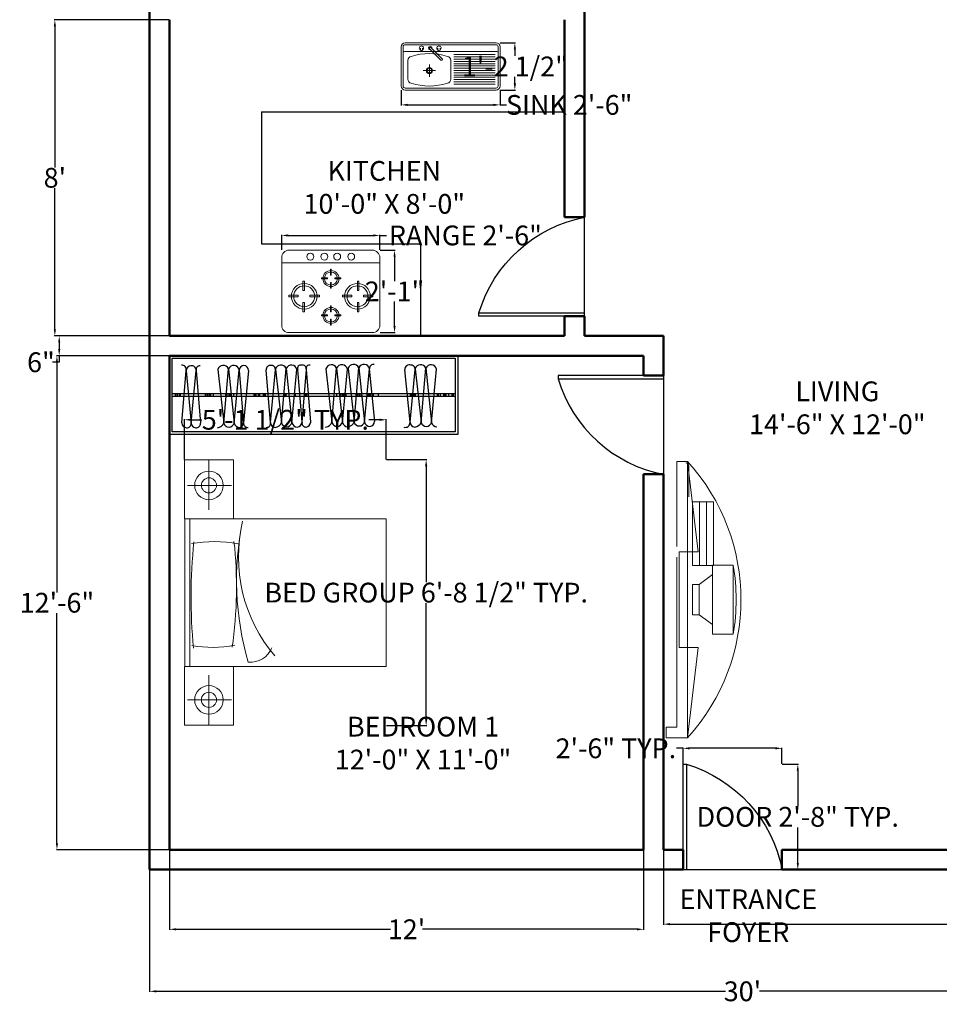
# Model space of a CAD drawing. Units: inches. Extents: x 20 to 32681, y 45 to 3082.
# Tile 1 of 5: x 21 to 301, y 45 to 344. Entities that reach past the tile are written whole.
import ezdxf

# ---------------------------------------------------------------- set-up
doc = ezdxf.new("R2010")
doc.units = ezdxf.units.IN
doc.header["$MEASUREMENT"] = 0
for name, color, linetype, lineweight in [('A-ANNO-DIMS', 2, 'Continuous', 18), ('A-AREA-IDEN', 7, 'Continuous', 25), ('A-DOOR', 4, 'Continuous', 25), ('A-EQPM', 9, 'Continuous', 18), ('A-FLOR-CASE', 32, 'Continuous', 25), ('A-FLOR-FIXT', 8, 'Continuous', 18), ('A-FURN', 8, 'Continuous', 18), ('A-WALL', 7, 'Continuous', 50)]:
    doc.layers.add(name, color=color, linetype=linetype, lineweight=lineweight)
doc.styles.get("Standard").update_dxf_attribs({"font": 'arial.ttf'})
doc.dimstyles.get("Standard").update_dxf_attribs({"dimtxt": 6, "dimasz": 2, "dimexe": 0.18, "dimexo": 0.0625, "dimgap": 0.09, "dimtad": 0, "dimtih": 1, "dimtoh": 1, "dimdec": 0, "dimzin": 0, "dimdsep": 46, "dimlunit": 4, "dimtxsty": 'Standard', "dimcen": 0.09, "dimadec": 0, "dimazin": 0, "dimtfac": 1, "dimtdec": 0, "dimtofl": 0, "dimtmove": 0, "dimatfit": 3, "dimfxl": 1, "dimtolj": 1, "dimtzin": 0, "dimarcsym": 0})

# ---------------------------------------------------------------- blocks, each defined once
blk = doc.blocks.new('DOOR')
for p, q in [((234.79, 441.58), (233.79, 441.58)), ((233.79, 441.58), (233.79, 409.58)), ((234.79, 409.58), (234.79, 441.58)), ((234.79, 409.58), (204.79, 409.58))]:
    blk.add_line(p, q)
blk.add_arc((245.82, 401.53), 41.82, 106.7253, 168.9058)
blk = doc.blocks.new('CVBN')
for p, q in [((70.94, 1179.16), (70.94, 1191.01)), ((89.36, 1192.66), (89.36, 1168.36)), ((89.36, 1081.69), (89.36, 1192.39)), ((89.36, 1192.39), (89.36, 1168.09)), ((170.36, 1192.39), (89.36, 1192.39)), ((170.36, 1192.66), (170.36, 1168.36)), ((170.36, 1081.69), (170.36, 1192.39)), ((170.36, 1192.39), (170.36, 1168.09)), ((170.36, 1192.39), (170.36, 1168.09)), ((188.79, 1179.16), (188.79, 1191.01)), ((170.36, 1189.69), (89.36, 1189.69)), ((70.94, 1179.16), (56.8, 1179.16)), ((70.94, 1179.16), (84.43, 1179.16)), ((70.94, 1179.16), (70.94, 1166.85)), ((188.79, 1179.16), (175.29, 1179.16)), ((188.79, 1179.16), (202.93, 1179.16)), ((188.79, 1179.16), (188.79, 1166.85)), ((170.36, 1081.69), (89.36, 1081.69))]:
    blk.add_line(p, q)
for points in [[(56.96, 1192.66), (56.96, 1165.66), (89.36, 1165.66), (89.36, 1192.66)], [(202.76, 1192.66), (202.76, 1165.66), (170.36, 1165.66), (170.36, 1192.66)]]:
    blk.add_lwpolyline(points, close=True)
for centre, radius in [((70.94, 1179.16), 7.85), ((188.79, 1179.16), 7.85), ((70.94, 1179.16), 4.15), ((188.79, 1179.16), 4.15)]:
    blk.add_circle(centre, radius)
for centre, radius, start, end in [((127.34, 900.05), 288.94, 83.953, 95.5626), ((165.23, 1177.16), 65.44, 169.9145, 190.6851), ((88.06, 1176.29), 69.84, 349.1761, 10.2706), ((136.55, 1004.48), 159.53, 78.2462, 106.3473), ((132.8, 1394.24), 230.23, 261.7649, 276.2896), ((149.51, 1078.87), 84.09, 76.5636, 130.3236), ((104.49, 1156.51), 12.88, 175.3269, 247.5588)]:
    blk.add_arc(centre, radius, start, end)
blk = doc.blocks.new('A$C025C2FF6')
for p, q in [((45, 500), (550, 500)), ((0, 45), (0, 455)), ((295.2, 454.2), (300.9, 454.2)), ((295.2, 418.5), (295.2, 454.2)), ((300.9, 418.5), (295.2, 418.5)), ((300.9, 454.2), (300.9, 418.5)), ((595, 455), (595, 45)), ((128.2, 316.3), (128.2, 373.4)), ((128.2, 373.4), (137.4, 373.4)), ((137.4, 373.4), (137.4, 316.3)), ((241.9, 397.2), (241.9, 391.5)), ((277.6, 397.2), (241.9, 397.2)), ((241.9, 391.5), (277.6, 391.5)), ((277.6, 391.5), (277.6, 397.2)), ((295.2, 374), (295.2, 338.4)), ((300.9, 374), (295.2, 374)), ((300.9, 338.4), (300.9, 374)), ((322.1, 397.2), (357.7, 397.2)), ((322.1, 391.5), (322.1, 397.2)), ((357.7, 391.5), (322.1, 391.5)), ((357.7, 397.2), (357.7, 391.5)), ((467.8, 373.4), (458.7, 373.4)), ((458.7, 373.4), (458.7, 316.3)), ((467.8, 316.3), (467.8, 373.4)), ((137.4, 316.3), (128.2, 316.3)), ((295.2, 338.4), (300.9, 338.4)), ((458.7, 316.3), (467.8, 316.3)), ((100.1, 282.2), (43, 282.2)), ((43, 282.2), (43, 273.1)), ((43, 273.1), (100.1, 273.1)), ((100.1, 273.1), (100.1, 282.2)), ((128.2, 245.2), (128.2, 188.1)), ((137.4, 245.2), (128.2, 245.2)), ((137.4, 188.1), (137.4, 245.2)), ((171.3, 282.2), (228.3, 282.2)), ((171.3, 273.1), (171.3, 282.2)), ((228.3, 273.1), (171.3, 273.1)), ((228.3, 282.2), (228.3, 273.1)), ((367.8, 282.2), (367.8, 273.1)), ((424.8, 282.2), (367.8, 282.2)), ((367.8, 273.1), (424.8, 273.1)), ((424.8, 273.1), (424.8, 282.2)), ((458.7, 188.1), (458.7, 245.2)), ((458.7, 245.2), (467.8, 245.2)), ((467.8, 245.2), (467.8, 188.1)), ((496, 273.1), (496, 282.2)), ((496, 282.2), (553, 282.2)), ((553, 273.1), (496, 273.1)), ((553, 282.2), (553, 273.1)), ((128.2, 188.1), (137.4, 188.1)), ((295.2, 195.2), (295.2, 230.9)), ((295.2, 230.9), (300.9, 230.9)), ((300.9, 195.2), (295.2, 195.2)), ((300.9, 230.9), (300.9, 195.2)), ((467.8, 188.1), (458.7, 188.1)), ((277.6, 173.9), (241.9, 173.9)), ((241.9, 173.9), (241.9, 168.2)), ((241.9, 168.2), (277.6, 168.2)), ((277.6, 168.2), (277.6, 173.9)), ((300.9, 150.7), (295.2, 150.7)), ((295.2, 150.7), (295.2, 115.1)), ((300.9, 115.1), (300.9, 150.7)), ((322.1, 168.2), (322.1, 173.9)), ((322.1, 173.9), (357.7, 173.9)), ((357.7, 168.2), (322.1, 168.2)), ((357.7, 173.9), (357.7, 168.2)), ((1.2, 76.7), (594.9, 76.7)), ((295.2, 115.1), (300.9, 115.1)), ((550, 0), (45, 0))]:
    blk.add_line(p, q)
at = {"extrusion": (1e-16, 1e-16, -1)}
for centre, start_param, end_param in [((45, 455), 3.926991, 5.497787), ((550, 45), 0.785398, 2.356194)]:
    blk.add_ellipse(centre, major_axis=(31.8, 31.8), ratio=1, start_param=start_param, end_param=end_param, dxfattribs=at)
at = {"extrusion": (0, 0, -1)}
for centre, start_param, end_param in [((550, 455), 0.785398, 2.356194), ((45, 45), 3.926991, 5.497787)]:
    blk.add_ellipse(centre, major_axis=(-31.8, 31.8), ratio=1, start_param=start_param, end_param=end_param, dxfattribs=at)
at = {"extrusion": (1e-16, 3e-16, -1)}
for centre in [(298.7, 395.6), (298.7, 172.3)]:
    blk.add_ellipse(centre, major_axis=(-34.4, 34.4), ratio=1, start_param=5.497787, end_param=11.780972, dxfattribs=at)
at = {"extrusion": (1e-16, 2e-16, -1)}
for centre in [(298.7, 395.6), (298.7, 172.3)]:
    blk.add_ellipse(centre, major_axis=(-28.1, 28.1), ratio=1, start_param=5.497787, end_param=11.780972, dxfattribs=at)
at = {"extrusion": (-1e-16, -1e-16, -1)}
blk.add_ellipse((136.5, 279.7), major_axis=(-55.1, 55.1), ratio=1, start_param=5.497787, end_param=11.780972, dxfattribs=at)
at = {"extrusion": (0, -4e-16, -1)}
blk.add_ellipse((136.5, 279.7), major_axis=(-44.9, 44.9), ratio=1, start_param=5.497787, end_param=11.780972, dxfattribs=at)
for centre, major_axis, start_param, end_param in [((459.5, 279.7), (55.1, 55.1), 5.497787, 11.780972), ((459.5, 279.7), (44.9, 44.9), 5.497787, 11.780972), ((336.3, 39), (-14.8, 14.8), 3.926991, 10.210176), ((421.3, 39), (-14.8, 14.8), 3.926991, 10.210176)]:
    blk.add_ellipse(centre, major_axis=major_axis, ratio=1, start_param=start_param, end_param=end_param)
at = {"extrusion": (2e-16, -1e-16, -1)}
for centre in [(173.7, 39), (258.7, 39)]:
    blk.add_ellipse(centre, major_axis=(14.8, 14.8), ratio=1, start_param=3.926991, end_param=10.210176, dxfattribs=at)
blk = doc.blocks.new('A$C24281843')
for p, q in [((0, 0.742), (0, 0.067)), ((1.626, 0.81), (0.067, 0.81)), ((0.067, 0.776), (1.626, 0.776)), ((0.328, 0.681), (0.328, 0.718)), ((0.366, 0.681), (0.366, 0.718)), ((0.487, 0.708), (0.681, 0.514)), ((0.701, 0.534), (0.507, 0.728)), ((0.628, 0.681), (0.628, 0.718)), ((0.666, 0.681), (0.666, 0.718)), ((1.693, 0.067), (1.693, 0.742)), ((1.637, 0.66), (0.056, 0.66)), ((0.134, 0.66), (0.056, 0.66)), ((0.115, 0.508), (0.115, 0.186)), ((0.85, 0.186), (0.85, 0.508)), ((0.902, 0.607), (1.607, 0.607)), ((0.902, 0.568), (1.607, 0.568)), ((0.902, 0.529), (1.607, 0.529)), ((0.482, 0.439), (0.482, 0.224)), ((0.902, 0.49), (1.607, 0.49)), ((0.902, 0.451), (1.607, 0.451)), ((0.902, 0.412), (1.607, 0.412)), ((0.902, 0.373), (1.607, 0.373)), ((0.375, 0.332), (0.59, 0.332)), ((0.902, 0.334), (1.607, 0.334)), ((0.902, 0.296), (1.607, 0.296)), ((0.902, 0.257), (1.607, 0.257)), ((0.902, 0.218), (1.607, 0.218)), ((0.902, 0.179), (1.607, 0.179)), ((0.067, 0.034), (1.626, 0.034)), ((0.902, 0.14), (1.607, 0.14)), ((0.902, 0.101), (1.607, 0.101)), ((1.626, 0), (0.067, 0))]:
    blk.add_line(p, q)
for points in [[(0.034, 0.742), (0.034, 0.067)], [(1.66, 0.067), (1.66, 0.742)]]:
    blk.add_lwpolyline(points)
for points in [[(0.172, 0.576, -0.154641), (0.792, 0.576)], [(0.172, 0.117, 0.154641), (0.792, 0.117, -0.022148)]]:
    blk.add_lwpolyline(points, format="xyb")
for radius in [0.0538, 0.0403]:
    blk.add_circle((0.482, 0.332), radius)
for centre, radius, start, end in [((0.067, 0.742), 0.0675, 90, 180), ((0.067, 0.742), 0.0338, 90, 180), ((0.347, 0.718), 0.0375, 300, 240), ((0.347, 0.706), 0.0318, 233.9153, 306.0847), ((0.497, 0.718), 0.0281, 345, 285), ((0.497, 0.718), 0.0141, 45, 225), ((0.647, 0.718), 0.0375, 300, 240), ((0.647, 0.706), 0.0318, 233.9153, 306.0847), ((1.626, 0.742), 0.0675, 0, 90), ((1.626, 0.742), 0.0338, 0, 90), ((0.056, 0.637), 0.0225, 90, 180), ((0.184, 0.508), 0.07, 100.6708, 179.5694), ((0.691, 0.524), 0.0141, 225, 45), ((0.78, 0.508), 0.07, 0.4306, 79.3292), ((1.637, 0.637), 0.0225, 0, 90), ((0.184, 0.186), 0.07, 180.4306, 259.3292), ((0.78, 0.186), 0.07, 280.6708, 359.5694), ((0.067, 0.067), 0.0675, 180, 270), ((0.067, 0.067), 0.0338, 180, 270), ((1.626, 0.067), 0.0675, 270, 0), ((1.626, 0.067), 0.0338, 270, 0)]:
    blk.add_arc(centre, radius, start, end)
blk = doc.blocks.new('A$C1DC223CE')
for p, q in [((0, 600, -1028.6), (2200, 600, -1028.6)), ((0, 0, -1028.6), (0, 600, -1028.6)), ((20, 580, -1028.6), (2180, 580, -1028.6)), ((20, 20, -1028.6), (20, 580, -1028.6)), ((2180, 580, -1028.6), (2180, 20, -1028.6)), ((2200, 600, -1028.6), (2200, 0, -1028.6)), ((94.7, 87.9, -1028.6), (127.5, 487.8, -1028.6)), ((127.7, 485.6, -1028.6), (166.3, 85.2, -1028.6)), ((165.4, 87.9, -1028.6), (203.9, 488.4, -1028.6)), ((203.9, 488.4, -1028.6), (236.8, 85.2, -1028.6)), ((369, 495.3, -1028.6), (414.4, 87.9, -1028.6)), ((414.4, 85.2, -1028.6), (450.2, 500.8, -1028.6)), ((450.2, 499.4, -1028.6), (494.2, 86.5, -1028.6)), ((494.2, 85.2, -1028.6), (532.8, 491.1, -1028.6)), ((532.8, 488.4, -1028.6), (565.6, 84.9, -1028.6)), ((604.3, 488.4, -1028.6), (565.8, 87.9, -1028.6)), ((770.7, 91.2, -1028.6), (737.6, 491.1, -1028.6)), ((770.7, 90.7, -1028.6), (809.2, 491.1, -1028.6)), ((809.2, 498, -1028.6), (854.6, 90.7, -1028.6)), ((854.6, 87.9, -1028.6), (890.4, 503.5, -1028.6)), ((890.4, 502.1, -1028.6), (934.4, 89.3, -1028.6)), ((934.4, 87.9, -1028.6), (973, 493.9, -1028.6)), ((1011.5, 93.4, -1028.6), (978.9, 493.9, -1028.6)), ((1011.5, 93.2, -1028.6), (1044.5, 493.9, -1028.6)), ((1077.5, 93.4, -1028.6), (1044.9, 493.9, -1028.6)), ((1193.8, 500.5, -1028.6), (1239.2, 93.1, -1028.6)), ((1239.2, 90.4, -1028.6), (1275, 506, -1028.6)), ((1275, 504.6, -1028.6), (1319, 91.8, -1028.6)), ((1319, 90.4, -1028.6), (1357.6, 496.4, -1028.6)), ((1363.1, 503.2, -1028.6), (1408.5, 95.9, -1028.6)), ((1408.5, 93.1, -1028.6), (1444.3, 508.7, -1028.6)), ((1444.3, 507.4, -1028.6), (1488.3, 94.5, -1028.6)), ((1488.3, 93.1, -1028.6), (1526.8, 499.1, -1028.6)), ((1565.4, 98.6, -1028.6), (1526.8, 499.1, -1028.6)), ((1835.1, 92.3, -1028.6), (1794.6, 493.3, -1028.6)), ((1835.1, 93.1, -1028.6), (1873.6, 493.6, -1028.6)), ((1873.6, 500.5, -1028.6), (1919, 93.1, -1028.6)), ((1919, 90.4, -1028.6), (1954.8, 506, -1028.6)), ((1954.8, 504.6, -1028.6), (1998.8, 91.8, -1028.6)), ((1998.8, 90.4, -1028.6), (2037.4, 496.4, -1028.6)), ((2180, 309.1, -1028.6), (20, 309.1, -1028.6)), ((44.6, 309.1, -1028.6), (44.6, 288.1, -1028.6)), ((50, 309.1, -1028.6), (50, 288.1, -1028.6)), ((62.8, 309.1, -1028.6), (62.8, 288.1, -1028.6)), ((77.5, 309.1, -1028.6), (77.5, 288.1, -1028.6)), ((82.9, 309.1, -1028.6), (82.9, 288.1, -1028.6)), ((272.7, 309.1, -1028.6), (272.7, 288.1, -1028.6)), ((278.2, 309.1, -1028.6), (278.2, 288.1, -1028.6)), ((291, 309.1, -1028.6), (291, 288.1, -1028.6)), ((303.7, 309.1, -1028.6), (303.7, 288.1, -1028.6)), ((312.9, 309.1, -1028.6), (312.9, 288.1, -1028.6)), ((333, 309.1, -1028.6), (333, 288.1, -1028.6)), ((427.5, 309.1, -1028.6), (427.5, 288.1, -1028.6)), ((433, 309.1, -1028.6), (433, 288.1, -1028.6)), ((445.8, 309.1, -1028.6), (445.8, 288.1, -1028.6)), ((458.6, 309.1, -1028.6), (458.6, 288.1, -1028.6)), ((467.7, 309.1, -1028.6), (467.7, 288.1, -1028.6)), ((487.8, 309.1, -1028.6), (487.8, 288.1, -1028.6)), ((644.9, 309.1, -1028.6), (644.9, 288.1, -1028.6)), ((650.4, 309.1, -1028.6), (650.4, 288.1, -1028.6)), ((659.5, 309.1, -1028.6), (659.5, 288.1, -1028.6)), ((677.8, 309.1, -1028.6), (677.8, 288.1, -1028.6)), ((683.3, 309.1, -1028.6), (683.3, 288.1, -1028.6)), ((686.9, 309.1, -1028.6), (686.9, 288.1, -1028.6)), ((716.2, 309.1, -1028.6), (716.2, 288.1, -1028.6)), ((725.3, 309.1, -1028.6), (725.3, 288.1, -1028.6)), ((730.8, 309.1, -1028.6), (730.8, 288.1, -1028.6)), ((876.9, 309.1, -1028.6), (876.9, 288.1, -1028.6)), ((887.9, 309.1, -1028.6), (887.9, 288.1, -1028.6)), ((951.8, 309.1, -1028.6), (951.8, 288.1, -1028.6)), ((959.1, 309.1, -1028.6), (959.1, 288.1, -1028.6)), ((1035.8, 309.1, -1028.6), (1035.8, 288.1, -1028.6)), ((1046.8, 309.1, -1028.6), (1046.8, 288.1, -1028.6)), ((1273.3, 309.1, -1028.6), (1273.3, 288.1, -1028.6)), ((1308, 309.1, -1028.6), (1308, 288.1, -1028.6)), ((1318.9, 309.1, -1028.6), (1318.9, 288.1, -1028.6)), ((1329.9, 309.1, -1028.6), (1329.9, 288.1, -1028.6)), ((1340.9, 309.1, -1028.6), (1340.9, 288.1, -1028.6)), ((1346.3, 309.1, -1028.6), (1346.3, 288.1, -1028.6)), ((1421.1, 309.1, -1028.6), (1421.1, 288.1, -1028.6)), ((1432.3, 309.1, -1028.6), (1432.3, 288.1, -1028.6)), ((1445.6, 309.1, -1028.6), (1445.6, 288.1, -1028.6)), ((1447.9, 309.1, -1028.6), (1447.9, 288.1, -1028.6)), ((1459, 309.1, -1028.6), (1459, 288.1, -1028.6)), ((1465.7, 309.1, -1028.6), (1465.7, 288.1, -1028.6)), ((1512.6, 309.1, -1028.6), (1512.6, 288.1, -1028.6)), ((1521.5, 309.1, -1028.6), (1521.5, 288.1, -1028.6)), ((1531.8, 309.1, -1028.6), (1531.8, 288.1, -1028.6)), ((1543.8, 309.1, -1028.6), (1543.8, 288.1, -1028.6)), ((1552.7, 309.1, -1028.6), (1552.7, 288.1, -1028.6)), ((1592, 309.1, -1028.6), (1592, 288.1, -1028.6)), ((1835.6, 309.1, -1028.6), (1835.6, 288.1, -1028.6)), ((1843.6, 309.1, -1028.6), (1843.6, 288.1, -1028.6)), ((1855.7, 309.1, -1028.6), (1855.7, 288.1, -1028.6)), ((1865.1, 309.1, -1028.6), (1865.1, 288.1, -1028.6)), ((1874.4, 309.1, -1028.6), (1874.4, 288.1, -1028.6)), ((2043.1, 309.1, -1028.6), (2043.1, 288.1, -1028.6)), ((2048.4, 309.1, -1028.6), (2048.4, 288.1, -1028.6)), ((2065.8, 309.1, -1028.6), (2065.8, 288.1, -1028.6)), ((2091.3, 309.1, -1028.6), (2091.3, 288.1, -1028.6)), ((2099.3, 309.1, -1028.6), (2099.3, 288.1, -1028.6)), ((2108.7, 309.1, -1028.6), (2108.7, 288.1, -1028.6)), ((2127.4, 309.1, -1028.6), (2127.4, 288.1, -1028.6)), ((2152.9, 309.1, -1028.6), (2152.9, 288.1, -1028.6)), ((2163.6, 309.1, -1028.6), (2163.6, 288.1, -1028.6)), ((2180, 288.1, -1028.6), (20, 288.1, -1028.6)), ((2200, 0, -1028.6), (0, 0, -1028.6)), ((2180, 20, -1028.6), (20, 20, -1028.6))]:
    blk.add_line(p, q)
for centre, radius, start, end in [((97.7, 496.3, -1028.6), 31, 344.07456, 99.05003), ((410.7, 482.3, -1028.6), 43.6, 25.03177, 162.72523), ((490.2, 482.2, -1028.6), 43.5, 11.80451, 156.77437), ((571.2, 487.1, -1028.6), 38.5, 94.01528, 178.14652), ((565.8, 487.1, -1028.6), 38.5, 1.85348, 85.98472), ((769.2, 494.1, -1028.6), 31.7, 82.36762, 185.38571), ((777.6, 494.1, -1028.6), 31.7, 354.61429, 97.63238), ((850.8, 485.1, -1028.6), 43.6, 25.03177, 162.72523), ((930.4, 485, -1028.6), 43.5, 11.80451, 156.77437), ((1002.3, 503.7, -1028.6), 25.4, 75.27133, 202.7917), ((1012.9, 496.9, -1028.6), 31.7, 354.61429, 97.63238), ((1068.3, 503.7, -1028.6), 25.4, 75.27133, 202.7917), ((1235.5, 487.5, -1028.6), 43.6, 25.03177, 162.72523), ((1315, 487.5, -1028.6), 43.5, 11.80451, 156.77437), ((1404.7, 490.3, -1028.6), 43.6, 25.03177, 162.72523), ((1484.2, 490.2, -1028.6), 43.5, 11.80451, 156.77437), ((1558.4, 502.1, -1028.6), 31.7, 82.36762, 185.38571), ((1830.5, 493.8, -1028.6), 35.9, 71.18865, 180.69602), ((1842, 496.6, -1028.6), 31.7, 354.61429, 97.63238), ((1915.3, 487.5, -1028.6), 43.6, 25.03177, 162.72523), ((1994.8, 487.5, -1028.6), 43.5, 11.80451, 156.77437), ((166.2, 484.4, -1028.6), 38.5, 94.01528, 178.14652), ((171.3, 490.9, -1028.6), 32.8, 355.49469, 103.64775), ((232.3, 493.9, -1028.6), 29, 86.55737, 190.95766), ((133.2, 89.2, -1028.6), 38.5, 181.85348, 265.98472), ((134.7, 82.2, -1028.6), 31.7, 262.36762, 5.38571), ((203.9, 89.2, -1028.6), 38.5, 181.85348, 265.98472), ((205.3, 82.2, -1028.6), 31.7, 262.36762, 5.38571), ((364, 103.5, -1028.6), 52.8, 272.47718, 342.81801), ((454.1, 97.9, -1028.6), 41.7, 197.75037, 344.22518), ((535.5, 96.3, -1028.6), 42.8, 195.04774, 270), ((528.6, 90.3, -1028.6), 37.5, 280.6806, 351.72432), ((597.4, 84.9, -1028.6), 31.7, 174.61429, 277.63238), ((741.6, 83.6, -1028.6), 30.1, 267.73367, 14.61166), ((809.1, 91.9, -1028.6), 38.5, 181.85348, 265.98472), ((804.2, 106.3, -1028.6), 52.8, 272.47718, 342.81801), ((894.3, 100.6, -1028.6), 41.7, 197.75037, 344.22518), ((975.7, 99, -1028.6), 42.8, 195.04774, 270), ((973, 94.7, -1028.6), 38.5, 274.01528, 358.14652), ((1040.4, 86.1, -1028.6), 29.8, 166.12938, 272.54601), ((1039.1, 94.7, -1028.6), 38.5, 274.01528, 358.14652), ((1188.8, 108.7, -1028.6), 52.8, 272.47718, 342.81801), ((1278.9, 103.1, -1028.6), 41.7, 197.75037, 344.22518), ((1360.3, 101.5, -1028.6), 42.8, 195.04774, 270), ((1358, 111.5, -1028.6), 52.8, 272.47718, 342.81801), ((1448.2, 105.8, -1028.6), 41.7, 197.75037, 344.22518), ((1529.6, 104.2, -1028.6), 42.8, 195.04774, 270), ((1526.9, 99.9, -1028.6), 38.5, 274.01528, 358.14652), ((1799, 89.7, -1028.6), 36.2, 250.23449, 4.119), ((1873.6, 94.4, -1028.6), 38.5, 181.85348, 265.98472), ((1868.6, 108.7, -1028.6), 52.8, 272.47718, 342.81801), ((1958.7, 103.1, -1028.6), 41.7, 197.75037, 344.22518), ((2040.1, 101.5, -1028.6), 42.8, 195.04774, 270)]:
    blk.add_arc(centre, radius, start, end)
blk = doc.blocks.new('*D16')
at = {"layer": 'A-ANNO-DIMS', "color": 0, "lineweight": -2, "transparency": 16777216}
for p, q in [((66.73, 343.58), (31.84, 343.58)), ((32.02, 341.58), (32.02, 298.73)), ((32.02, 249.58), (32.02, 292.42)), ((66.73, 247.58), (31.84, 247.58))]:
    blk.add_line(p, q, dxfattribs=at)
at = {"layer": 'A-ANNO-DIMS', "color": 0, "transparency": 16777216}
for points in [[(31.69, 341.58), (32.35, 341.58), (32.02, 343.58)], [(31.69, 249.58), (32.35, 249.58), (32.02, 247.58)]]:
    blk.add_solid(points, dxfattribs=at)
at = {"layer": 'Defpoints', "color": 0, "transparency": 16777216}
for p in [(66.79, 343.58), (32.02, 247.58), (66.79, 247.58)]:
    blk.add_point(p, dxfattribs=at)
at = {"layer": 'A-ANNO-DIMS', "color": 0, "transparency": 16777216, "insert": (32.02, 295.58), "char_height": 6, "attachment_point": 5}
blk.add_mtext("\\A1;8'", dxfattribs=at)
blk = doc.blocks.new('*D17')
at = {"layer": 'A-ANNO-DIMS', "color": 0, "lineweight": -2, "transparency": 16777216}
for p, q in [((66.73, 241.58), (32.47, 241.58)), ((32.65, 239.58), (32.65, 169.73)), ((32.65, 93.58), (32.65, 163.42)), ((66.73, 91.58), (32.47, 91.58))]:
    blk.add_line(p, q, dxfattribs=at)
at = {"layer": 'A-ANNO-DIMS', "color": 0, "transparency": 16777216}
for points in [[(32.32, 239.58), (32.99, 239.58), (32.65, 241.58)], [(32.32, 93.58), (32.99, 93.58), (32.65, 91.58)]]:
    blk.add_solid(points, dxfattribs=at)
at = {"layer": 'Defpoints', "color": 0, "transparency": 16777216}
for p in [(66.79, 241.58), (32.65, 91.58), (66.79, 91.58)]:
    blk.add_point(p, dxfattribs=at)
at = {"layer": 'A-ANNO-DIMS', "color": 0, "transparency": 16777216, "insert": (32.65, 166.58), "char_height": 6, "attachment_point": 5}
blk.add_mtext('\\A1;12\'-6"', dxfattribs=at)
blk = doc.blocks.new('*D18')
at = {"layer": 'A-ANNO-DIMS', "color": 0, "lineweight": -2, "transparency": 16777216}
for p, q in [((66.73, 247.58), (33.16, 247.58)), ((33.34, 245.58), (33.34, 243.58)), ((33.34, 239.58), (31.34, 239.58)), ((66.73, 241.58), (33.16, 241.58)), ((33.34, 241.58), (33.34, 239.58))]:
    blk.add_line(p, q, dxfattribs=at)
at = {"layer": 'A-ANNO-DIMS', "color": 0, "transparency": 16777216}
for points in [[(33.01, 245.58), (33.68, 245.58), (33.34, 247.58)], [(33.01, 243.58), (33.68, 243.58), (33.34, 241.58)]]:
    blk.add_solid(points, dxfattribs=at)
at = {"layer": 'Defpoints', "color": 0, "transparency": 16777216}
for p in [(66.79, 247.58), (33.34, 241.58), (66.79, 241.58)]:
    blk.add_point(p, dxfattribs=at)
at = {"layer": 'A-ANNO-DIMS', "color": 0, "transparency": 16777216, "insert": (27.79, 239.58), "char_height": 6, "attachment_point": 5}
blk.add_mtext('\\A1;6"', dxfattribs=at)
blk = doc.blocks.new('*D19')
at = {"layer": 'A-ANNO-DIMS', "color": 0, "lineweight": -2, "transparency": 16777216}
for p, q in [((66.79, 91.51), (66.79, 67.26)), ((210.79, 91.51), (210.79, 67.26)), ((68.79, 67.44), (133.89, 67.44)), ((208.79, 67.44), (143.69, 67.44))]:
    blk.add_line(p, q, dxfattribs=at)
at = {"layer": 'A-ANNO-DIMS', "color": 0, "transparency": 16777216}
for points in [[(68.79, 67.77), (68.79, 67.11), (66.79, 67.44)], [(208.79, 67.77), (208.79, 67.11), (210.79, 67.44)]]:
    blk.add_solid(points, dxfattribs=at)
at = {"layer": 'Defpoints', "color": 0, "transparency": 16777216}
for p in [(66.79, 91.58), (210.79, 91.58), (210.79, 67.44)]:
    blk.add_point(p, dxfattribs=at)
at = {"layer": 'A-ANNO-DIMS', "color": 0, "transparency": 16777216, "insert": (138.79, 67.44), "char_height": 6, "attachment_point": 5}
blk.add_mtext("\\A1;12'", dxfattribs=at)
blk = doc.blocks.new('*D20')
at = {"layer": 'A-ANNO-DIMS', "color": 0, "lineweight": -2, "transparency": 16777216}
for p, q in [((216.79, 91.51), (216.79, 68.82)), ((414.79, 91.51), (414.79, 68.82)), ((218.79, 69), (305.68, 69)), ((412.79, 69), (325.9, 69))]:
    blk.add_line(p, q, dxfattribs=at)
at = {"layer": 'A-ANNO-DIMS', "color": 0, "transparency": 16777216}
for points in [[(218.79, 69.34), (218.79, 68.67), (216.79, 69)], [(412.79, 69.34), (412.79, 68.67), (414.79, 69)]]:
    blk.add_solid(points, dxfattribs=at)
at = {"layer": 'Defpoints', "color": 0, "transparency": 16777216}
for p in [(216.79, 91.58), (414.79, 91.58), (414.79, 69)]:
    blk.add_point(p, dxfattribs=at)
at = {"layer": 'A-ANNO-DIMS', "color": 0, "transparency": 16777216, "insert": (315.79, 69), "char_height": 6, "attachment_point": 5}
blk.add_mtext('\\A1;16\'-6"', dxfattribs=at)
blk = doc.blocks.new('*D27')
at = {"layer": 'A-ANNO-DIMS', "color": 0, "lineweight": -2, "transparency": 16777216}
for p, q in [((60.79, 85.51), (60.79, 48.43)), ((420.79, 85.51), (420.79, 48.43)), ((62.79, 48.61), (235.61, 48.61)), ((418.79, 48.61), (245.97, 48.61))]:
    blk.add_line(p, q, dxfattribs=at)
at = {"layer": 'A-ANNO-DIMS', "color": 0, "transparency": 16777216}
for points in [[(62.79, 48.94), (62.79, 48.27), (60.79, 48.61)], [(418.79, 48.94), (418.79, 48.27), (420.79, 48.61)]]:
    blk.add_solid(points, dxfattribs=at)
at = {"layer": 'Defpoints', "color": 0, "transparency": 16777216}
for p in [(60.79, 85.58), (420.79, 85.58), (420.79, 48.61)]:
    blk.add_point(p, dxfattribs=at)
at = {"layer": 'A-ANNO-DIMS', "color": 0, "transparency": 16777216, "insert": (240.79, 48.61), "char_height": 6, "attachment_point": 5}
blk.add_mtext("\\A1;30'", dxfattribs=at)
blk = doc.blocks.new('*D30')
at = {"layer": 'A-ANNO-DIMS', "color": 0, "lineweight": -2, "transparency": 16777216}
for p, q in [((252.85, 117.58), (257.77, 117.58)), ((257.59, 115.58), (257.59, 104.77)), ((257.59, 87.58), (257.59, 98.38)), ((252.85, 85.58), (257.77, 85.58))]:
    blk.add_line(p, q, dxfattribs=at)
at = {"layer": 'A-ANNO-DIMS', "color": 0, "transparency": 16777216}
for points in [[(257.26, 115.58), (257.92, 115.58), (257.59, 117.58)], [(257.26, 87.58), (257.92, 87.58), (257.59, 85.58)]]:
    blk.add_solid(points, dxfattribs=at)
at = {"layer": 'Defpoints', "color": 0, "transparency": 16777216}
for p in [(252.79, 117.58), (257.59, 117.58), (252.79, 85.58)]:
    blk.add_point(p, dxfattribs=at)
at = {"layer": 'A-ANNO-DIMS', "color": 0, "transparency": 16777216, "insert": (257.59, 101.58), "char_height": 6, "attachment_point": 5}
blk.add_mtext('\\A1;DOOR 2\'-8" TYP.', dxfattribs=at)
blk = doc.blocks.new('*D31')
at = {"layer": 'A-ANNO-DIMS', "color": 0, "lineweight": -2, "transparency": 16777216}
for p, q in [((222.79, 117.64), (222.79, 122.56)), ((252.79, 117.64), (252.79, 122.56)), ((222.79, 122.38), (220.79, 122.38)), ((250.79, 122.38), (224.79, 122.38))]:
    blk.add_line(p, q, dxfattribs=at)
at = {"layer": 'A-ANNO-DIMS', "color": 0, "transparency": 16777216}
for points in [[(224.79, 122.71), (224.79, 122.04), (222.79, 122.38)], [(250.79, 122.71), (250.79, 122.04), (252.79, 122.38)]]:
    blk.add_solid(points, dxfattribs=at)
at = {"layer": 'Defpoints', "color": 0, "transparency": 16777216}
for p in [(222.79, 122.38), (222.79, 117.58), (252.79, 117.58)]:
    blk.add_point(p, dxfattribs=at)
at = {"layer": 'A-ANNO-DIMS', "color": 0, "transparency": 16777216, "insert": (202.36, 122.38), "char_height": 6, "attachment_point": 5}
blk.add_mtext('\\A1;2\'-6" TYP.', dxfattribs=at)
blk = doc.blocks.new('*D32')
at = {"layer": 'A-ANNO-DIMS', "color": 0, "lineweight": -2, "transparency": 16777216}
for p, q in [((132.72, 210.01), (144.94, 210.01)), ((144.76, 208.01), (144.76, 172.84)), ((144.76, 131.28), (144.76, 166.45)), ((132.72, 129.28), (144.94, 129.28))]:
    blk.add_line(p, q, dxfattribs=at)
at = {"layer": 'A-ANNO-DIMS', "color": 0, "transparency": 16777216}
for points in [[(144.43, 208.01), (145.1, 208.01), (144.76, 210.01)], [(144.43, 131.28), (145.1, 131.28), (144.76, 129.28)]]:
    blk.add_solid(points, dxfattribs=at)
at = {"layer": 'Defpoints', "color": 0, "transparency": 16777216}
for p in [(132.65, 210.01), (144.76, 210.01), (132.65, 129.28)]:
    blk.add_point(p, dxfattribs=at)
at = {"layer": 'A-ANNO-DIMS', "color": 0, "transparency": 16777216, "insert": (144.76, 169.65), "char_height": 6, "attachment_point": 5}
blk.add_mtext('\\A1;BED GROUP 6\'-8 1/2" TYP.', dxfattribs=at)
blk = doc.blocks.new('*D33')
at = {"layer": 'A-ANNO-DIMS', "color": 0, "lineweight": -2, "transparency": 16777216}
for p, q in [((71.35, 210.08), (71.35, 222.3)), ((73.35, 222.12), (76.63, 222.12)), ((130.65, 222.12), (127.37, 222.12)), ((132.65, 210.08), (132.65, 222.3))]:
    blk.add_line(p, q, dxfattribs=at)
at = {"layer": 'A-ANNO-DIMS', "color": 0, "transparency": 16777216}
for points in [[(73.35, 222.46), (73.35, 221.79), (71.35, 222.12)], [(130.65, 222.46), (130.65, 221.79), (132.65, 222.12)]]:
    blk.add_solid(points, dxfattribs=at)
at = {"layer": 'Defpoints', "color": 0, "transparency": 16777216}
for p in [(71.35, 222.12), (71.35, 210.01), (132.65, 210.01)]:
    blk.add_point(p, dxfattribs=at)
at = {"layer": 'A-ANNO-DIMS', "color": 0, "transparency": 16777216, "insert": (102, 222.12), "char_height": 6, "attachment_point": 5}
blk.add_mtext('\\A1;5\'-1 1/2" TYP.', dxfattribs=at)
blk = doc.blocks.new('*D40')
at = {"layer": 'A-ANNO-DIMS', "color": 0, "lineweight": -2, "transparency": 16777216}
for p, q in [((100.89, 273.67), (100.89, 278.26)), ((102.89, 278.08), (128.69, 278.08)), ((130.69, 273.67), (130.69, 278.26)), ((130.69, 278.08), (132.69, 278.08))]:
    blk.add_line(p, q, dxfattribs=at)
at = {"layer": 'A-ANNO-DIMS', "color": 0, "transparency": 16777216}
for points in [[(102.89, 278.41), (102.89, 277.75), (100.89, 278.08)], [(128.69, 278.41), (128.69, 277.75), (130.69, 278.08)]]:
    blk.add_solid(points, dxfattribs=at)
at = {"layer": 'Defpoints', "color": 0, "transparency": 16777216}
for p in [(130.69, 278.08), (100.89, 273.61), (130.69, 273.61)]:
    blk.add_point(p, dxfattribs=at)
at = {"layer": 'A-ANNO-DIMS', "color": 0, "transparency": 16777216, "insert": (156.67, 278.08), "char_height": 6, "attachment_point": 5}
blk.add_mtext('\\A1;RANGE 2\'-6"', dxfattribs=at)
blk = doc.blocks.new('*D41')
at = {"layer": 'A-ANNO-DIMS', "color": 0, "lineweight": -2, "transparency": 16777216}
for p, q in [((130.75, 273.61), (135.34, 273.61)), ((135.16, 271.61), (135.16, 264.19)), ((135.16, 250.57), (135.16, 257.99)), ((130.75, 248.57), (135.34, 248.57))]:
    blk.add_line(p, q, dxfattribs=at)
at = {"layer": 'A-ANNO-DIMS', "color": 0, "transparency": 16777216}
for points in [[(134.83, 271.61), (135.49, 271.61), (135.16, 273.61)], [(134.83, 250.57), (135.49, 250.57), (135.16, 248.57)]]:
    blk.add_solid(points, dxfattribs=at)
at = {"layer": 'Defpoints', "color": 0, "transparency": 16777216}
for p in [(130.69, 273.61), (130.69, 248.57), (135.16, 248.57)]:
    blk.add_point(p, dxfattribs=at)
at = {"layer": 'A-ANNO-DIMS', "color": 0, "transparency": 16777216, "insert": (135.16, 261.09), "char_height": 6, "attachment_point": 5}
blk.add_mtext('\\A1;2\'-1"', dxfattribs=at)
blk = doc.blocks.new('*D42')
at = {"layer": 'A-ANNO-DIMS', "color": 0, "lineweight": -2, "transparency": 16777216}
for p, q in [((137.18, 322.15), (137.18, 317.53)), ((167.19, 322.15), (167.19, 317.53)), ((139.18, 317.71), (165.19, 317.71)), ((167.19, 317.71), (169.19, 317.71))]:
    blk.add_line(p, q, dxfattribs=at)
at = {"layer": 'A-ANNO-DIMS', "color": 0, "transparency": 16777216}
for points in [[(139.18, 318.05), (139.18, 317.38), (137.18, 317.71)], [(165.19, 318.05), (165.19, 317.38), (167.19, 317.71)]]:
    blk.add_solid(points, dxfattribs=at)
at = {"layer": 'Defpoints', "color": 0, "transparency": 16777216}
for p in [(137.18, 322.22), (167.19, 322.22), (167.19, 317.71)]:
    blk.add_point(p, dxfattribs=at)
at = {"layer": 'A-ANNO-DIMS', "color": 0, "transparency": 16777216, "insert": (188.18, 317.71), "char_height": 6, "attachment_point": 5}
blk.add_mtext('\\A1;SINK 2\'-6"', dxfattribs=at)
blk = doc.blocks.new('*D43')
at = {"layer": 'A-ANNO-DIMS', "color": 0, "lineweight": -2, "transparency": 16777216}
for p, q in [((167.25, 336.57), (171.87, 336.57)), ((171.69, 334.57), (171.69, 332.59)), ((171.69, 324.22), (171.69, 326.2)), ((167.25, 322.22), (171.87, 322.22))]:
    blk.add_line(p, q, dxfattribs=at)
at = {"layer": 'A-ANNO-DIMS', "color": 0, "transparency": 16777216}
for points in [[(171.35, 334.57), (172.02, 334.57), (171.69, 336.57)], [(171.35, 324.22), (172.02, 324.22), (171.69, 322.22)]]:
    blk.add_solid(points, dxfattribs=at)
at = {"layer": 'Defpoints', "color": 0, "transparency": 16777216}
for p in [(167.19, 336.57), (171.69, 336.57), (167.19, 322.22)]:
    blk.add_point(p, dxfattribs=at)
at = {"layer": 'A-ANNO-DIMS', "color": 0, "transparency": 16777216, "insert": (171.69, 329.39), "char_height": 6, "attachment_point": 5}
blk.add_mtext('\\A1;1\'-2 1/2"', dxfattribs=at)

msp = doc.modelspace()

# ---------------------------------------------------------------- linework, layer by layer
at = {"layer": 'A-FLOR-CASE'}
for p, q in [((94.79, 315.58), (186.79, 315.58)), ((94.79, 315.58), (94.79, 275.58)), ((94.79, 275.58), (143.05, 275.58)), ((143.05, 275.58), (143.05, 247.58))]:
    msp.add_line(p, q, dxfattribs=at)
at = {"layer": 'A-FURN'}
for p, q in [((220.89, 183.64), (220.89, 209.43)), ((224.12, 209.43), (220.89, 209.43)), ((224.12, 125.61), (224.12, 209.43)), ((227.34, 182.03), (224.12, 209.43)), ((225.59, 177.91), (225.59, 197.24)), ((225.59, 197.24), (232.04, 197.24)), ((227.72, 197.24), (227.72, 177.91)), ((229.91, 197.24), (229.91, 177.91)), ((232.04, 197.24), (232.04, 177.91)), ((220.89, 128.84), (220.89, 180.42)), ((221.54, 153.01), (221.54, 182.03)), ((221.54, 182.03), (227.34, 182.03)), ((232.04, 177.91), (225.59, 177.91)), ((231.69, 157.07), (231.69, 177.98)), ((231.69, 177.98), (238.02, 177.98)), ((238.02, 157.07), (238.02, 177.98)), ((231.69, 175.12), (227.68, 172.15)), ((225.64, 172.15), (225.64, 162.9)), ((227.68, 172.15), (225.64, 172.15)), ((227.68, 172.15), (227.68, 162.9)), ((227.68, 162.9), (225.64, 162.9)), ((231.69, 159.93), (227.68, 162.9)), ((231.69, 157.07), (238.02, 157.07)), ((221.54, 153.01), (227.34, 153.01)), ((227.34, 153.01), (224.12, 125.61)), ((217.67, 125.61), (217.67, 128.84)), ((220.89, 128.84), (217.67, 128.84)), ((224.12, 125.61), (217.67, 125.61))]:
    msp.add_line(p, q, dxfattribs=at)
for points in [[(224.12, 125.61, 0.386509), (224.12, 209.43, -2.260033)], [(223.57, 209.02, -0.414214), (224.47, 208.11), (224.47, 198.72)]]:
    msp.add_lwpolyline(points, format="xyb", dxfattribs=at)
msp.add_arc((174.21, 167.52), 64.66, 350.6925, 9.3075, dxfattribs=at)
at = {"layer": 'A-WALL'}
for p, q in [((60.79, 565.58), (60.79, 85.58)), ((192.79, 349.58), (192.79, 283.58)), ((66.79, 343.58), (66.79, 247.58)), ((186.79, 343.58), (186.79, 283.58)), ((186.79, 283.58), (192.79, 283.58)), ((186.79, 253.58), (192.79, 253.58)), ((186.79, 253.58), (186.79, 247.58)), ((192.79, 253.58), (192.79, 247.58)), ((66.79, 247.58), (186.79, 247.58)), ((192.79, 247.58), (216.79, 247.58)), ((216.79, 247.58), (216.79, 235.58)), ((66.79, 241.58), (210.79, 241.58)), ((66.79, 241.58), (66.79, 91.58)), ((210.79, 241.58), (210.79, 235.58)), ((210.79, 235.58), (216.79, 235.58)), ((210.79, 205.58), (216.79, 205.58)), ((210.79, 205.58), (210.79, 91.58)), ((216.79, 205.58), (216.79, 91.58)), ((66.79, 91.58), (210.79, 91.58)), ((216.79, 91.58), (222.79, 91.58)), ((222.79, 91.58), (222.79, 85.58)), ((252.79, 91.58), (252.79, 85.58)), ((252.79, 91.58), (414.79, 91.58)), ((60.79, 85.58), (222.79, 85.58)), ((252.79, 85.58), (420.79, 85.58))]:
    msp.add_line(p, q, dxfattribs=at)

# ---------------------------------------------------------------- block references
at = {"layer": 'A-DOOR', "xscale": -1, "rotation": 90}
msp.add_blockref('DOOR', (602.37, 488.37), dxfattribs=at)
at = {"layer": 'A-DOOR', "rotation": 90}
msp.add_blockref('DOOR', (626.37, 0.78), dxfattribs=at)
at = {"layer": 'A-DOOR', "xscale": -1}
msp.add_blockref('DOOR', (457.58, -324), dxfattribs=at)
at = {"layer": 'A-EQPM', "xscale": -0.0500853766148243, "yscale": 0.0500853766148243, "zscale": 0.0500853766148243, "rotation": 180}
msp.add_blockref('A$C025C2FF6', (100.89, 273.61), dxfattribs=at)
at = {"layer": 'A-FLOR-CASE', "xscale": 0.039818128500731, "yscale": 0.039818128500731, "zscale": 0.039818128500731}
msp.add_blockref('A$C1DC223CE', (66.79, 217.68, 40.96), dxfattribs=at)
at = {"layer": 'A-FLOR-FIXT', "xscale": 17.72298413343992, "yscale": 17.72298413343992, "zscale": 17.72298413343992}
msp.add_blockref('A$C24281843', (137.18, 322.22), dxfattribs=at)
at = {"layer": 'A-FURN', "xscale": 0.55247276188645, "yscale": 0.55247276188645, "zscale": 0.55247276188645, "rotation": 90}
msp.add_blockref('CVBN', (730.26, 97.9), dxfattribs=at)

# ---------------------------------------------------------------- texts
at = {"layer": 'A-AREA-IDEN', "char_height": 6, "attachment_point": 1}
for s, width, insert in [('\\pxqc;KITCHEN\\P10\'-0" X 8\'-0"', 130.2327, (66.93, 300.67)), ('\\pxqc;LIVING\\P14\'-6" X 12\'-0"', 89.6456, (224.77, 233.75)), ('\\pxqc;BEDROOM 1\\P12\'-0" X 11\'-0"', 119.244, (84.18, 131.96)), ('\\pxqc;ENTRANCE\\PFOYER', 88.7208, (198.19, 79.57))]:
    msp.add_mtext_dynamic_manual_height_columns(s, width=width, gutter_width=30, heights=[0], dxfattribs=dict(at, insert=insert))

# ---------------------------------------------------------------- dimensions: what is measured, and where the dimension line sits
at = {"layer": 'A-ANNO-DIMS'}
for base, p1, p2, angle, override, picture, middle in [((32.02, 247.58), (66.79, 343.58), (66.79, 247.58), 90, {"dimclrd": 0, "dimclre": 0, "dimclrt": 0}, '*D16', (32.02, 295.58)), ((171.6867, 336.5714), (167.1852, 322.2157), (167.1852, 336.5714), 90, {"dimdec": 1, "dimlfac": 1, "dimrnd": 0, "dimzin": 1, "dimdsep": 46, "dimlunit": 4, "dimfrac": 2}, '*D43', (171.6867, 329.3935)), ((135.16, 248.57), (130.69, 273.61), (130.69, 248.57), 270, {"dimdec": 1, "dimlfac": 1, "dimrnd": 0, "dimzin": 1, "dimdsep": 46, "dimlunit": 4, "dimfrac": 2}, '*D41', (135.16, 261.09)), ((33.34, 241.58), (66.79, 247.58), (66.79, 241.58), 90, {"dimclrd": 0, "dimclre": 0, "dimclrt": 0}, '*D18', (27.79, 239.58)), ((32.65, 91.58), (66.79, 241.58), (66.79, 91.58), 90, {"dimclrd": 0, "dimclre": 0, "dimclrt": 0}, '*D17', (32.65, 166.58))]:
    dim = msp.add_linear_dim(base=base, p1=p1, p2=p2, angle=angle, dimstyle='Standard', override=override, dxfattribs=at)
    dim.commit()
    dim.dimension.update_dxf_attribs({"geometry": picture, "text_midpoint": middle})
for base, p1, p2, text, picture, middle in [((167.19, 317.71), (137.18, 322.22), (167.19, 322.22), 'SINK <>', '*D42', (188.18, 317.71)), ((130.69, 278.08), (100.89, 273.61), (130.69, 273.61), 'RANGE <>', '*D40', (156.67, 278.08))]:
    dim = msp.add_linear_dim(base=base, p1=p1, p2=p2, text=text, dimstyle='Standard', override={"dimdec": 1, "dimlfac": 1, "dimrnd": 0, "dimzin": 1, "dimdsep": 46, "dimlunit": 4, "dimfrac": 2}, dxfattribs=at)
    dim.commit()
    dim.dimension.update_dxf_attribs({"geometry": picture, "text_midpoint": middle})
for base, p1, p2, angle, text, picture, middle in [((71.35, 222.12), (132.65, 210.01), (71.35, 210.01), 180, '<> TYP.', '*D33', (102, 222.12)), ((144.76, 210.01), (132.65, 129.28), (132.65, 210.01), 90, 'BED GROUP <> TYP.', '*D32', (144.76, 169.65)), ((222.79, 122.38), (252.79, 117.58), (222.79, 117.58), 180, '<> TYP.', '*D31', (202.36, 122.38)), ((257.59, 117.58), (252.79, 85.58), (252.79, 117.58), 90, 'DOOR <> TYP.', '*D30', (257.59, 101.58))]:
    dim = msp.add_linear_dim(base=base, p1=p1, p2=p2, angle=angle, text=text, dimstyle='Standard', override={"dimdec": 1, "dimlfac": 1, "dimrnd": 0, "dimzin": 1, "dimdsep": 46, "dimlunit": 4, "dimfrac": 2}, dxfattribs=at)
    dim.commit()
    dim.dimension.update_dxf_attribs({"geometry": picture, "text_midpoint": middle})
for base, p1, p2, picture, middle in [((210.79, 67.44), (66.79, 91.58), (210.79, 91.58), '*D19', (138.79, 67.44)), ((414.79, 69), (216.79, 91.58), (414.79, 91.58), '*D20', (315.79, 69)), ((420.79, 48.61), (60.79, 85.58), (420.79, 85.58), '*D27', (240.79, 48.61))]:
    dim = msp.add_linear_dim(base=base, p1=p1, p2=p2, dimstyle='Standard', override={"dimclrd": 0, "dimclre": 0, "dimclrt": 0}, dxfattribs=at)
    dim.commit()
    dim.dimension.update_dxf_attribs({"geometry": picture, "text_midpoint": middle})

doc.saveas('drawing.dxf')
